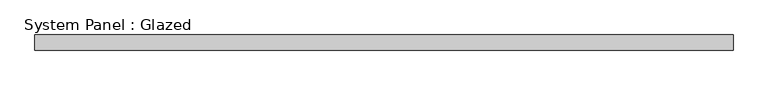
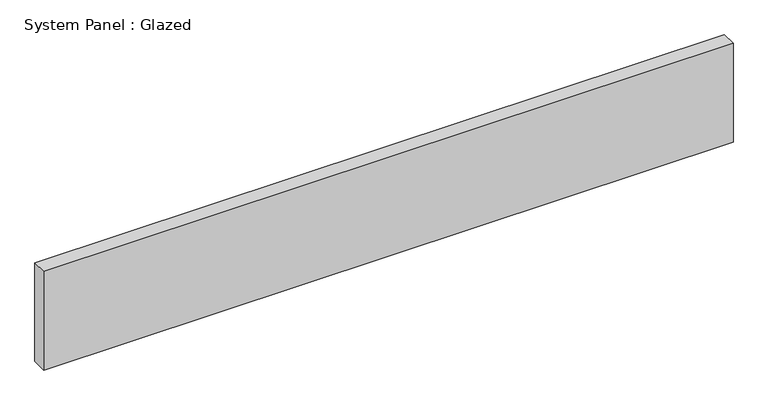
"""IFC4 building model written with IfcOpenShell, lengths in millimetres: plate geometry, System Panel : Glazed."""

from ifc_helpers import new_model, si_unit, origin, origin_with_axes, place, context, project, spatial, polyline, outline, extrude, source, transform, mapped, element, save


def system_panel_glazed_cafbbc3c(model_context):
    return source(origin(), model_context, "Body", "SweptSolid", [
        extrude(outline(polyline([(587.3750001, 19.05), (-587.3750001, 19.05), (-587.3750001, 44.45), (587.3750001, 44.45), (587.3750001, 19.05)])), origin_with_axes(), (0.0, 0.0, 1.0), 177.8),
    ])


if __name__ == "__main__":
    model = new_model("IFC4")
    model_context = context("Model", 3, world=origin())
    ifc_project = project(units=[si_unit("LENGTHUNIT", "METRE", prefix="MILLI")], contexts=[model_context])
    site = spatial("IfcSite", under=ifc_project)
    building = spatial("IfcBuilding", under=site)
    placement = place(None, origin())
    system_panel_glazed_shape = system_panel_glazed_cafbbc3c(model_context)
    element("IfcPlate", 1, ObjectType="System Panel : Glazed", at=placement, inside=building, context=model_context, shape_type="MappedRepresentation", body=[
        mapped(system_panel_glazed_shape, transform((0.0, 0.0, 0.0), x_axis=(1.0, 0.0, 0.0), y_axis=(0.0, 1.0, 0.0), z_axis=(0.0, 0.0, 1.0))),
    ])
    save(model, "model.ifc")

# Revit data of these elements
# Type "System Panel : Glazed"
#   Construction Type Id = "GSP4R"
#   Analytic Construction = "1/8 in Pilkington single glazing"
#   Visual Light Transmittance = 0.9
#   Solar Heat Gain Coefficient = 0.86
#   Heat Transfer Coefficient (U) = 1.18115 BTU/(h·ft²·°F)
#   Define Thermal Properties by = 1
# Element 1 (IfcPlate, "System Panel : Glazed")
#   Materials on its faces: "Glass"
# Materials
#   "Glass": class "Glass", colour RGB 0 128 192, transparency 0.75, Description = "Soda Lime Glass", Cost = 0
